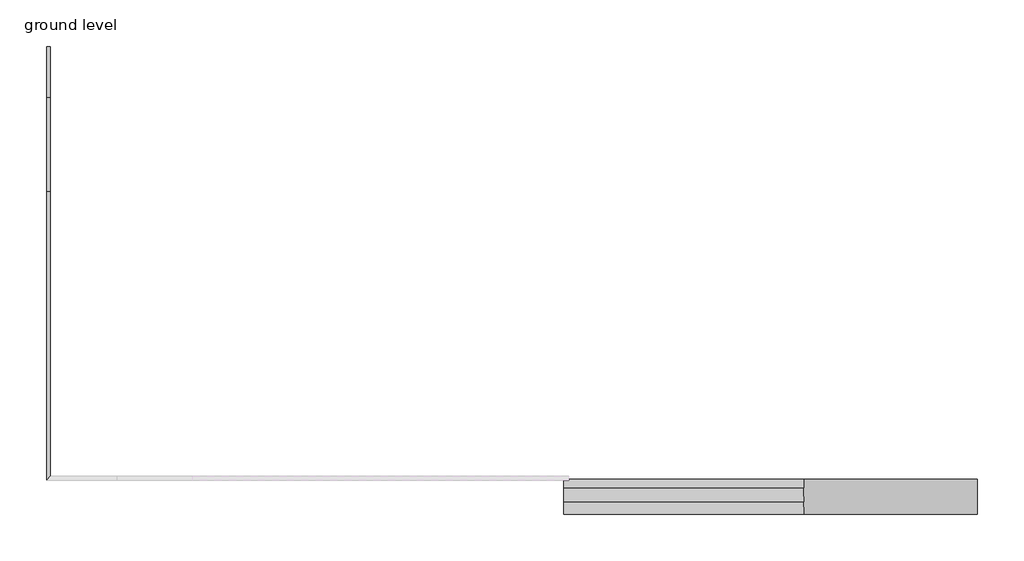
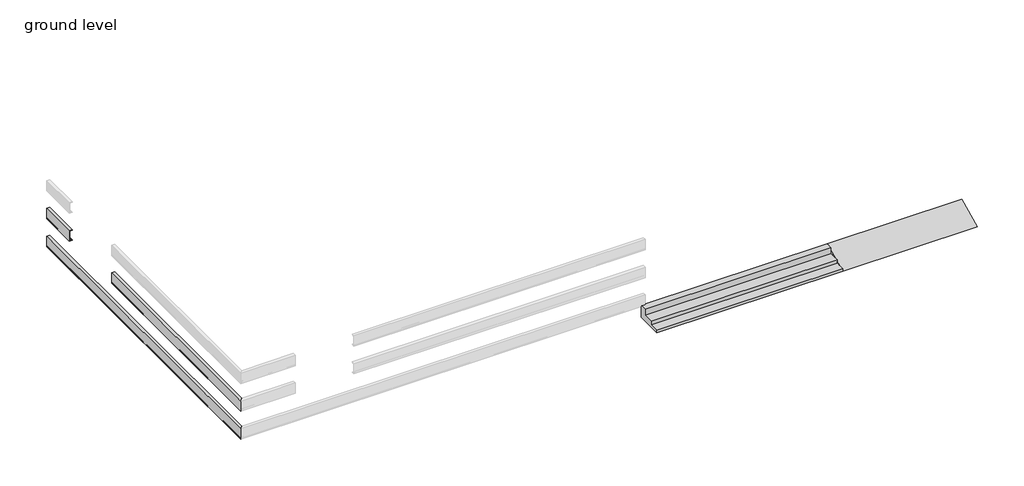
# One storey, part 3 of 3: 4 proxies.
"""IFC4 building model written with IfcOpenShell, lengths in millimetres."""

from ifc_helpers import new_model, si_unit, frame, origin, place, context, project, spatial, polyline, circle_curve, ellipse_curve, transform, mapped, element, save
from ifc_brep_helpers import plane_surface, cylinder_surface, revolved_surface, advanced_brep
from components import generic_models_3_generic_models_3_935cad4b, generic_models_4_generic_models_4_8b3ef071

model = new_model("IFC4")

# Units and contexts
model_context = context("Model", 3, world=origin())
ifc_project = project(units=[si_unit("LENGTHUNIT", "METRE", prefix="MILLI")], contexts=[model_context])

# Site, building, storey
site = spatial("IfcSite", under=ifc_project)
building = spatial("IfcBuilding", under=site)
storey = spatial("IfcBuildingStorey", under=building, Name="ground level", Elevation=0.0)

# Proxies
placement = place(None, origin())
generic_models_3_generic_models_3_shape = generic_models_3_generic_models_3_935cad4b(model_context)
element("IfcBuildingElementProxy", 1, Name="Generic Models 3 : Generic Models 3", ObjectType="Generic Models 3 : Generic Models 3", at=placement, inside=storey, context=model_context, shape_type="MappedRepresentation", body=[
    mapped(generic_models_3_generic_models_3_shape, transform((0.0, 0.0, 0.0), x_axis=(1.0, 0.0, 0.0), y_axis=(0.0, 1.0, 0.0), z_axis=(0.0, 0.0, 1.0))),
])
generic_models_4_generic_models_4_shape = generic_models_4_generic_models_4_8b3ef071(model_context)
element("IfcBuildingElementProxy", 2, Name="Generic Models 4 : Generic Models 4", ObjectType="Generic Models 4 : Generic Models 4", at=placement, inside=storey, context=model_context, shape_type="MappedRepresentation", body=[
    mapped(generic_models_4_generic_models_4_shape, transform((0.0, 0.0, 0.0), x_axis=(1.0, 0.0, 0.0), y_axis=(0.0, 1.0, 0.0), z_axis=(0.0, 0.0, 1.0))),
])
element("IfcBuildingElementProxy", 3, Name="Reveal", ObjectType="Reveal", at=placement, inside=storey, context=model_context, shape_type="AdvancedBrep", body=[
    advanced_brep(
    [(-10842.2672301, -7280.1146427, 1079.5), (-10842.2672301, -7216.8686427, 1079.5), (-10842.2672301, -7216.8686427, 1078.1203242), (-10842.2672301, -7221.2514519, 1072.9465897), (-10842.2672301, -7244.8721427, 1069.0098), (-10842.2672301, -7264.1100243, 1065.80348), (-10842.2672301, -7272.8756427, 1055.456011), (-10842.2672301, -7272.8756427, 874.943989), (-10842.2672301, -7264.1100243, 864.59652), (-10842.2672301, -7244.8721427, 861.3902), (-10842.2672301, -7221.2514519, 857.4534103), (-10842.2672301, -7216.8686427, 852.2796758), (-10842.2672301, -7216.8686427, 850.9), (-10842.2672301, -7280.1146427, 850.9), (-4797.0672301, -7280.1146427, 1079.5), (-4797.0672301, -7280.1146427, 850.9), (-4797.0672301, -7216.8686427, 850.9), (-4797.0672301, -7216.8686427, 852.2796758), (-4797.0672301, -7221.2514519, 857.4534103), (-4797.0672301, -7244.8721427, 861.3902), (-4797.0672301, -7264.1100243, 864.59652), (-4797.0672301, -7272.8756427, 874.943989), (-4797.0672301, -7272.8756427, 1055.456011), (-4797.0672301, -7264.1100243, 1065.80348), (-4797.0672301, -7244.8721427, 1069.0098), (-4797.0672301, -7221.2514519, 1072.9465897), (-4797.0672301, -7216.8686427, 1078.1203242), (-4797.0672301, -7216.8686427, 1079.5)],
    [
        (0, 1),
        (1, 2),
        (2, 3, circle_curve(frame((-10842.2672301, -7222.1137427, 1078.1203242), z_axis=(-1.0, 0.0, 0.0), x_axis=(0.0, 1.0, 0.0)), 5.2451)),
        (3, 4),
        (4, 5),
        (5, 6, circle_curve(frame((-10842.2672301, -7262.3854427, 1055.456011), z_axis=(1.0, 0.0, 0.0), x_axis=(0.0, 1.0, 0.0)), 10.4902)),
        (6, 7),
        (7, 8, circle_curve(frame((-10842.2672301, -7262.3854427, 874.943989), z_axis=(1.0, 0.0, 0.0), x_axis=(0.0, 1.0, 0.0)), 10.4902)),
        (8, 9),
        (9, 10),
        (10, 11, circle_curve(frame((-10842.2672301, -7222.1137427, 852.2796758), z_axis=(-1.0, 0.0, 0.0), x_axis=(0.0, 1.0, 0.0)), 5.2451)),
        (11, 12),
        (12, 13),
        (13, 0),
        (14, 15),
        (15, 16),
        (16, 17),
        (17, 18, circle_curve(frame((-4797.0672301, -7222.1137427, 852.2796758), z_axis=(1.0, 0.0, 0.0), x_axis=(0.0, 1.0, 0.0)), 5.2451)),
        (18, 19),
        (19, 20),
        (20, 21, circle_curve(frame((-4797.0672301, -7262.3854427, 874.943989), z_axis=(-1.0, 0.0, 0.0), x_axis=(0.0, 1.0, 0.0)), 10.4902)),
        (21, 22),
        (22, 23, circle_curve(frame((-4797.0672301, -7262.3854427, 1055.456011), z_axis=(-1.0, 0.0, 0.0), x_axis=(0.0, 1.0, 0.0)), 10.4902)),
        (23, 24),
        (24, 25),
        (25, 26, circle_curve(frame((-4797.0672301, -7222.1137427, 1078.1203242), z_axis=(1.0, 0.0, 0.0), x_axis=(0.0, 1.0, 0.0)), 5.2451)),
        (26, 27),
        (27, 14),
        (0, 14),
        (27, 1),
        (26, 2),
        (25, 3),
        (24, 4),
        (23, 5),
        (22, 6),
        (21, 7),
        (20, 8),
        (19, 9),
        (18, 10),
        (17, 11),
        (16, 12),
        (15, 13),
    ],
    [
        plane_surface(frame((-10842.2672301, -7036.6302427, 914.4), z_axis=(-1.0, 0.0, 0.0), x_axis=(0.0, -1.0, 0.0))),
        plane_surface(frame((-4797.0672301, -7265.2302427, 841.0898298), z_axis=(1.0, 0.0, 0.0), x_axis=(0.0, 1.0, 0.0))),
        plane_surface(frame((-10842.2672301, -7280.1146427, 1079.5), z_axis=(0.0, 0.0, 1.0), x_axis=(1.0, 0.0, 0.0))),
        plane_surface(frame((-10842.2672301, -7216.8686427, 1079.5), z_axis=(0.0, 1.0, 0.0), x_axis=(1.0, 0.0, 0.0))),
        cylinder_surface(frame((-10842.2672301, -7222.1137427, 1078.1203242), z_axis=(-1.0, 0.0, 0.0), x_axis=(0.0, 1.0, 0.0)), 5.2451),
        plane_surface(frame((-10842.2672301, -7221.2514519, 1072.9465897), z_axis=(0.0, 0.16439930721687082, -0.9863938705135049), x_axis=(1.0, 0.0, 0.0))),
        plane_surface(frame((-10842.2672301, -7244.8721427, 1069.0098), z_axis=(0.0, 0.16439930721687146, -0.9863938705135048), x_axis=(1.0, 0.0, 0.0))),
        revolved_surface(polyline([(-4797.0672301, -7251.8952426999995, 1055.456011), (-10842.2672301, -7251.8952426999995, 1055.456011)]), (-10842.2672301, -7262.3854427, 1055.456011), (1.0, 0.0, 0.0)),
        plane_surface(frame((-10842.2672301, -7272.8756427, 1055.456011), z_axis=(0.0, 1.0, 0.0), x_axis=(1.0, 0.0, 0.0))),
        revolved_surface(polyline([(-4797.0672301, -7251.8952426999995, 874.943989), (-10842.2672301, -7251.8952426999995, 874.943989)]), (-10842.2672301, -7262.3854427, 874.943989), (1.0, 0.0, 0.0)),
        plane_surface(frame((-10842.2672301, -7264.1100243, 864.59652), z_axis=(0.0, 0.1643993072168769, 0.9863938705135039), x_axis=(1.0, 0.0, 0.0))),
        plane_surface(frame((-10842.2672301, -7244.8721427, 861.3902), z_axis=(0.0, 0.16439930721687793, 0.9863938705135037), x_axis=(1.0, 0.0, 0.0))),
        cylinder_surface(frame((-10842.2672301, -7222.1137427, 852.2796758), z_axis=(-1.0, 0.0, 0.0), x_axis=(0.0, 1.0, 0.0)), 5.2451),
        plane_surface(frame((-10842.2672301, -7216.8686427, 852.2796758), z_axis=(0.0, 1.0, 0.0), x_axis=(1.0, 0.0, 0.0))),
        plane_surface(frame((-10842.2672301, -7216.8686427, 850.9), z_axis=(0.0, 0.0, -1.0), x_axis=(1.0, 0.0, 0.0))),
        plane_surface(frame((-10842.2672301, -7280.1146427, 850.9), z_axis=(0.0, -1.0, 0.0), x_axis=(1.0, 0.0, 0.0))),
    ],
    [
        (0, [[1, 2, 3, 4, 5, 6, 7, 8, 9, 10, 11, 12, 13, 14]]),
        (1, [[15, 16, 17, 18, 19, 20, 21, 22, 23, 24, 25, 26, 27, 28]]),
        (2, [[-1, 29, -28, 30]]),
        (3, [[-2, -30, -27, 31]]),
        (4, [[-3, -31, -26, 32]]),
        (5, [[-4, -32, -25, 33]]),
        (6, [[-5, -33, -24, 34]]),
        (7, [[-6, -34, -23, 35]]),
        (8, [[-7, -35, -22, 36]]),
        (9, [[-8, -36, -21, 37]]),
        (10, [[-9, -37, -20, 38]]),
        (11, [[-10, -38, -19, 39]]),
        (12, [[-11, -39, -18, 40]]),
        (13, [[-12, -40, -17, 41]]),
        (14, [[-13, -41, -16, 42]]),
        (15, [[-14, -42, -15, -29]]),
    ],
),
    advanced_brep(
    [(-13193.9516301, -7280.1146427, 1079.5), (-13130.7056301, -7216.8686427, 1079.5), (-13130.7056301, -7216.8686427, 1078.1203242), (-13135.0884393, -7221.2514519, 1072.9465897), (-13158.7091301, -7244.8721427, 1069.0098), (-13177.9470117, -7264.1100243, 1065.80348), (-13186.7126301, -7272.8756427, 1055.456011), (-13186.7126301, -7272.8756427, 874.943989), (-13177.9470117, -7264.1100243, 864.59652), (-13158.7091301, -7244.8721427, 861.3902), (-13135.0884393, -7221.2514519, 857.4534103), (-13130.7056301, -7216.8686427, 852.2796758), (-13130.7056301, -7216.8686427, 850.9), (-13193.9516301, -7280.1146427, 850.9), (-12061.4672301, -7280.1146427, 1079.5), (-12061.4672301, -7280.1146427, 850.9), (-12061.4672301, -7216.8686427, 850.9), (-12061.4672301, -7216.8686427, 852.2796758), (-12061.4672301, -7221.2514519, 857.4534103), (-12061.4672301, -7244.8721427, 861.3902), (-12061.4672301, -7264.1100243, 864.59652), (-12061.4672301, -7272.8756427, 874.943989), (-12061.4672301, -7272.8756427, 1055.456011), (-12061.4672301, -7264.1100243, 1065.80348), (-12061.4672301, -7244.8721427, 1069.0098), (-12061.4672301, -7221.2514519, 1072.9465897), (-12061.4672301, -7216.8686427, 1078.1203242), (-12061.4672301, -7216.8686427, 1079.5)],
    [
        (0, 1),
        (1, 2),
        (2, 3, ellipse_curve(frame((-13135.9507301, -7222.1137427, 1078.1203242), z_axis=(-0.7071067811865476, 0.7071067811865476, 0.0), x_axis=(-0.7071067811865475, -0.7071067811865476, 0.0)), 7.4176916, 5.2451)),
        (3, 4),
        (4, 5),
        (5, 6, ellipse_curve(frame((-13176.2224301, -7262.3854427, 1055.456011), z_axis=(0.7071067811865476, -0.7071067811865476, 0.0), x_axis=(0.7071067811865475, 0.7071067811865476, 0.0)), 14.8353831, 10.4902)),
        (6, 7),
        (7, 8, ellipse_curve(frame((-13176.2224301, -7262.3854427, 874.943989), z_axis=(0.7071067811865476, -0.7071067811865476, 0.0), x_axis=(0.7071067811865475, 0.7071067811865476, 0.0)), 14.8353831, 10.4902)),
        (8, 9),
        (9, 10),
        (10, 11, ellipse_curve(frame((-13135.9507301, -7222.1137427, 852.2796758), z_axis=(-0.7071067811865476, 0.7071067811865476, 0.0), x_axis=(-0.7071067811865475, -0.7071067811865476, 0.0)), 7.4176916, 5.2451)),
        (11, 12),
        (12, 13),
        (13, 0),
        (14, 15),
        (15, 16),
        (16, 17),
        (17, 18, circle_curve(frame((-12061.4672301, -7222.1137427, 852.2796758), z_axis=(1.0, 0.0, 0.0), x_axis=(0.0, 1.0, 0.0)), 5.2451)),
        (18, 19),
        (19, 20),
        (20, 21, circle_curve(frame((-12061.4672301, -7262.3854427, 874.943989), z_axis=(-1.0, 0.0, 0.0), x_axis=(0.0, 1.0, 0.0)), 10.4902)),
        (21, 22),
        (22, 23, circle_curve(frame((-12061.4672301, -7262.3854427, 1055.456011), z_axis=(-1.0, 0.0, 0.0), x_axis=(0.0, 1.0, 0.0)), 10.4902)),
        (23, 24),
        (24, 25),
        (25, 26, circle_curve(frame((-12061.4672301, -7222.1137427, 1078.1203242), z_axis=(1.0, 0.0, 0.0), x_axis=(0.0, 1.0, 0.0)), 5.2451)),
        (26, 27),
        (27, 14),
        (0, 14),
        (27, 1),
        (26, 2),
        (25, 3),
        (24, 4),
        (23, 5),
        (22, 6),
        (21, 7),
        (20, 8),
        (19, 9),
        (18, 10),
        (17, 11),
        (16, 12),
        (15, 13),
    ],
    [
        plane_surface(frame((-13179.0672301, -7265.2302427, 660.4), z_axis=(-0.7071067811865476, 0.7071067811865476, 0.0), x_axis=(0.7071067811865476, 0.7071067811865476, 0.0))),
        plane_surface(frame((-12061.4672301, -7036.6302427, 2184.4), z_axis=(1.0, 0.0, 0.0), x_axis=(0.0, -1.0, 0.0))),
        plane_surface(frame((-13193.9516301, -7280.1146427, 1079.5), z_axis=(0.0, 0.0, 1.0), x_axis=(1.0, 0.0, 0.0))),
        plane_surface(frame((-13130.7056301, -7216.8686427, 1079.5), z_axis=(0.0, 1.0, 0.0), x_axis=(1.0, 0.0, 0.0))),
        cylinder_surface(frame((-13179.0672301, -7222.1137427, 1078.1203242), z_axis=(-1.0, 0.0, 0.0), x_axis=(0.0, 1.0, 0.0)), 5.2451),
        plane_surface(frame((-13135.0884393, -7221.2514519, 1072.9465897), z_axis=(0.0, 0.16439930721687082, -0.9863938705135049), x_axis=(1.0, 0.0, 0.0))),
        plane_surface(frame((-13158.7091301, -7244.8721427, 1069.0098), z_axis=(0.0, 0.16439930721687146, -0.9863938705135048), x_axis=(1.0, 0.0, 0.0))),
        revolved_surface(polyline([(-12061.4672301, -7251.8952426999995, 1055.456011), (-13186.7126301, -7251.8952426999995, 1055.456011)]), (-13179.0672301, -7262.3854427, 1055.456011), (1.0, 0.0, 0.0)),
        plane_surface(frame((-13186.7126301, -7272.8756427, 1055.456011), z_axis=(0.0, 1.0, 0.0), x_axis=(1.0, 0.0, 0.0))),
        revolved_surface(polyline([(-12061.4672301, -7251.8952426999995, 874.943989), (-13186.7126301, -7251.8952426999995, 874.943989)]), (-13179.0672301, -7262.3854427, 874.943989), (1.0, 0.0, 0.0)),
        plane_surface(frame((-13177.9470117, -7264.1100243, 864.59652), z_axis=(0.0, 0.1643993072168769, 0.9863938705135039), x_axis=(1.0, 0.0, 0.0))),
        plane_surface(frame((-13158.7091301, -7244.8721427, 861.3902), z_axis=(0.0, 0.16439930721687793, 0.9863938705135037), x_axis=(1.0, 0.0, 0.0))),
        cylinder_surface(frame((-13179.0672301, -7222.1137427, 852.2796758), z_axis=(-1.0, 0.0, 0.0), x_axis=(0.0, 1.0, 0.0)), 5.2451),
        plane_surface(frame((-13130.7056301, -7216.8686427, 852.2796758), z_axis=(0.0, 1.0, 0.0), x_axis=(1.0, 0.0, 0.0))),
        plane_surface(frame((-13130.7056301, -7216.8686427, 850.9), z_axis=(0.0, 0.0, -1.0), x_axis=(1.0, 0.0, 0.0))),
        plane_surface(frame((-13193.9516301, -7280.1146427, 850.9), z_axis=(0.0, -1.0, 0.0), x_axis=(1.0, 0.0, 0.0))),
    ],
    [
        (0, [[1, 2, 3, 4, 5, 6, 7, 8, 9, 10, 11, 12, 13, 14]]),
        (1, [[15, 16, 17, 18, 19, 20, 21, 22, 23, 24, 25, 26, 27, 28]]),
        (2, [[-1, 29, -28, 30]]),
        (3, [[-2, -30, -27, 31]]),
        (4, [[-3, -31, -26, 32]]),
        (5, [[-4, -32, -25, 33]]),
        (6, [[-5, -33, -24, 34]]),
        (7, [[-6, -34, -23, 35]]),
        (8, [[-7, -35, -22, 36]]),
        (9, [[-8, -36, -21, 37]]),
        (10, [[-9, -37, -20, 38]]),
        (11, [[-10, -38, -19, 39]]),
        (12, [[-11, -39, -18, 40]]),
        (13, [[-12, -40, -17, 41]]),
        (14, [[-13, -41, -16, 42]]),
        (15, [[-14, -42, -15, -29]]),
    ],
),
    advanced_brep(
    [(-13193.9516301, -2642.4302427, 1079.5), (-13130.7056301, -2642.4302427, 1079.5), (-13130.7056301, -2642.4302427, 1078.1203242), (-13135.0884393, -2642.4302427, 1072.9465897), (-13158.7091301, -2642.4302427, 1069.0098), (-13177.9470117, -2642.4302427, 1065.80348), (-13186.7126301, -2642.4302427, 1055.456011), (-13186.7126301, -2642.4302427, 874.943989), (-13177.9470117, -2642.4302427, 864.59652), (-13158.7091301, -2642.4302427, 861.3902), (-13135.0884393, -2642.4302427, 857.4534103), (-13130.7056301, -2642.4302427, 852.2796758), (-13130.7056301, -2642.4302427, 850.9), (-13193.9516301, -2642.4302427, 850.9), (-13193.9516301, -7280.1146427, 1079.5), (-13193.9516301, -7280.1146427, 850.9), (-13130.7056301, -7216.8686427, 850.9), (-13130.7056301, -7216.8686427, 852.2796758), (-13135.0884393, -7221.2514519, 857.4534103), (-13158.7091301, -7244.8721427, 861.3902), (-13177.9470117, -7264.1100243, 864.59652), (-13186.7126301, -7272.8756427, 874.943989), (-13186.7126301, -7272.8756427, 1055.456011), (-13177.9470117, -7264.1100243, 1065.80348), (-13158.7091301, -7244.8721427, 1069.0098), (-13135.0884393, -7221.2514519, 1072.9465897), (-13130.7056301, -7216.8686427, 1078.1203242), (-13130.7056301, -7216.8686427, 1079.5)],
    [
        (0, 1),
        (1, 2),
        (2, 3, circle_curve(frame((-13135.9507301, -2642.4302427, 1078.1203242), z_axis=(0.0, 1.0, 0.0), x_axis=(1.0, 0.0, 0.0)), 5.2451)),
        (3, 4),
        (4, 5),
        (5, 6, circle_curve(frame((-13176.2224301, -2642.4302427, 1055.456011), z_axis=(0.0, -1.0, 0.0), x_axis=(1.0, 0.0, 0.0)), 10.4902)),
        (6, 7),
        (7, 8, circle_curve(frame((-13176.2224301, -2642.4302427, 874.943989), z_axis=(0.0, -1.0, 0.0), x_axis=(1.0, 0.0, 0.0)), 10.4902)),
        (8, 9),
        (9, 10),
        (10, 11, circle_curve(frame((-13135.9507301, -2642.4302427, 852.2796758), z_axis=(0.0, 1.0, 0.0), x_axis=(1.0, 0.0, 0.0)), 5.2451)),
        (11, 12),
        (12, 13),
        (13, 0),
        (14, 15),
        (15, 16),
        (16, 17),
        (17, 18, ellipse_curve(frame((-13135.9507301, -7222.1137427, 852.2796758), z_axis=(0.7071067811865476, -0.7071067811865476, 0.0), x_axis=(0.7071067811865477, 0.7071067811865474, 0.0)), 7.4176916, 5.2451)),
        (18, 19),
        (19, 20),
        (20, 21, ellipse_curve(frame((-13176.2224301, -7262.3854427, 874.943989), z_axis=(-0.7071067811865476, 0.7071067811865476, 0.0), x_axis=(-0.7071067811865477, -0.7071067811865474, 0.0)), 14.8353831, 10.4902)),
        (21, 22),
        (22, 23, ellipse_curve(frame((-13176.2224301, -7262.3854427, 1055.456011), z_axis=(-0.7071067811865476, 0.7071067811865476, 0.0), x_axis=(-0.7071067811865477, -0.7071067811865474, 0.0)), 14.8353831, 10.4902)),
        (23, 24),
        (24, 25),
        (25, 26, ellipse_curve(frame((-13135.9507301, -7222.1137427, 1078.1203242), z_axis=(0.7071067811865476, -0.7071067811865476, 0.0), x_axis=(0.7071067811865477, 0.7071067811865474, 0.0)), 7.4176916, 5.2451)),
        (26, 27),
        (27, 14),
        (0, 14),
        (27, 1),
        (26, 2),
        (25, 3),
        (24, 4),
        (23, 5),
        (22, 6),
        (21, 7),
        (20, 8),
        (19, 9),
        (18, 10),
        (17, 11),
        (16, 12),
        (15, 13),
    ],
    [
        plane_surface(frame((-12950.4672301, -2642.4302427, 914.4), z_axis=(0.0, 1.0, 0.0), x_axis=(-1.0, 0.0, 0.0))),
        plane_surface(frame((-13179.0672301, -7265.2302427, 660.4), z_axis=(0.7071067811865476, -0.7071067811865476, 0.0), x_axis=(0.7071067811865476, 0.7071067811865476, 0.0))),
        plane_surface(frame((-13193.9516301, -2642.4302427, 1079.5), z_axis=(0.0, 0.0, 1.0), x_axis=(0.0, -1.0, 0.0))),
        plane_surface(frame((-13130.7056301, -2642.4302427, 1079.5), z_axis=(1.0, 0.0, 0.0), x_axis=(0.0, -1.0, 0.0))),
        cylinder_surface(frame((-13135.9507301, -2642.4302427, 1078.1203242), z_axis=(0.0, 1.0, 0.0), x_axis=(1.0, 0.0, 0.0)), 5.2451),
        plane_surface(frame((-13135.0884393, -2642.4302427, 1072.9465897), z_axis=(0.16439930721687082, 0.0, -0.9863938705135049), x_axis=(0.0, -1.0, 0.0))),
        plane_surface(frame((-13158.7091301, -2642.4302427, 1069.0098), z_axis=(0.16439930721687146, 0.0, -0.9863938705135048), x_axis=(0.0, -1.0, 0.0))),
        revolved_surface(polyline([(-13165.7322301, -7272.875642700001, 1055.456011), (-13165.7322301, -2642.4302427, 1055.456011)]), (-13176.2224301, -2642.4302427, 1055.456011), (0.0, -1.0, 0.0)),
        plane_surface(frame((-13186.7126301, -2642.4302427, 1055.456011), z_axis=(1.0, 0.0, 0.0), x_axis=(0.0, -1.0, 0.0))),
        revolved_surface(polyline([(-13165.7322301, -7272.875642700001, 874.943989), (-13165.7322301, -2642.4302427, 874.943989)]), (-13176.2224301, -2642.4302427, 874.943989), (0.0, -1.0, 0.0)),
        plane_surface(frame((-13177.9470117, -2642.4302427, 864.59652), z_axis=(0.1643993072168769, 0.0, 0.9863938705135039), x_axis=(0.0, -1.0, 0.0))),
        plane_surface(frame((-13158.7091301, -2642.4302427, 861.3902), z_axis=(0.16439930721687793, 0.0, 0.9863938705135037), x_axis=(0.0, -1.0, 0.0))),
        cylinder_surface(frame((-13135.9507301, -2642.4302427, 852.2796758), z_axis=(0.0, 1.0, 0.0), x_axis=(1.0, 0.0, 0.0)), 5.2451),
        plane_surface(frame((-13130.7056301, -2642.4302427, 852.2796758), z_axis=(1.0, 0.0, 0.0), x_axis=(0.0, -1.0, 0.0))),
        plane_surface(frame((-13130.7056301, -2642.4302427, 850.9), z_axis=(0.0, 0.0, -1.0), x_axis=(0.0, -1.0, 0.0))),
        plane_surface(frame((-13193.9516301, -2642.4302427, 850.9), z_axis=(-1.0, 0.0, 0.0), x_axis=(0.0, -1.0, 0.0))),
    ],
    [
        (0, [[1, 2, 3, 4, 5, 6, 7, 8, 9, 10, 11, 12, 13, 14]]),
        (1, [[15, 16, 17, 18, 19, 20, 21, 22, 23, 24, 25, 26, 27, 28]]),
        (2, [[-1, 29, -28, 30]]),
        (3, [[-2, -30, -27, 31]]),
        (4, [[-3, -31, -26, 32]]),
        (5, [[-4, -32, -25, 33]]),
        (6, [[-5, -33, -24, 34]]),
        (7, [[-6, -34, -23, 35]]),
        (8, [[-7, -35, -22, 36]]),
        (9, [[-8, -36, -21, 37]]),
        (10, [[-9, -37, -20, 38]]),
        (11, [[-10, -38, -19, 39]]),
        (12, [[-11, -39, -18, 40]]),
        (13, [[-12, -40, -17, 41]]),
        (14, [[-13, -41, -16, 42]]),
        (15, [[-14, -42, -15, -29]]),
    ],
),
    advanced_brep(
    [(-13193.9516301, -305.6302427, 1079.5), (-13130.7056301, -305.6302427, 1079.5), (-13130.7056301, -305.6302427, 1078.1203242), (-13135.0884393, -305.6302427, 1072.9465897), (-13158.7091301, -305.6302427, 1069.0098), (-13177.9470117, -305.6302427, 1065.80348), (-13186.7126301, -305.6302427, 1055.456011), (-13186.7126301, -305.6302427, 874.943989), (-13177.9470117, -305.6302427, 864.59652), (-13158.7091301, -305.6302427, 861.3902), (-13135.0884393, -305.6302427, 857.4534103), (-13130.7056301, -305.6302427, 852.2796758), (-13130.7056301, -305.6302427, 850.9), (-13193.9516301, -305.6302427, 850.9), (-13193.9516301, -1118.4302427, 1079.5), (-13193.9516301, -1118.4302427, 850.9), (-13130.7056301, -1118.4302427, 850.9), (-13130.7056301, -1118.4302427, 852.2796758), (-13135.0884393, -1118.4302427, 857.4534103), (-13158.7091301, -1118.4302427, 861.3902), (-13177.9470117, -1118.4302427, 864.59652), (-13186.7126301, -1118.4302427, 874.943989), (-13186.7126301, -1118.4302427, 1055.456011), (-13177.9470117, -1118.4302427, 1065.80348), (-13158.7091301, -1118.4302427, 1069.0098), (-13135.0884393, -1118.4302427, 1072.9465897), (-13130.7056301, -1118.4302427, 1078.1203242), (-13130.7056301, -1118.4302427, 1079.5)],
    [
        (0, 1),
        (1, 2),
        (2, 3, circle_curve(frame((-13135.9507301, -305.6302427, 1078.1203242), z_axis=(0.0, 1.0, 0.0), x_axis=(1.0, 0.0, 0.0)), 5.2451)),
        (3, 4),
        (4, 5),
        (5, 6, circle_curve(frame((-13176.2224301, -305.6302427, 1055.456011), z_axis=(0.0, -1.0, 0.0), x_axis=(1.0, 0.0, 0.0)), 10.4902)),
        (6, 7),
        (7, 8, circle_curve(frame((-13176.2224301, -305.6302427, 874.943989), z_axis=(0.0, -1.0, 0.0), x_axis=(1.0, 0.0, 0.0)), 10.4902)),
        (8, 9),
        (9, 10),
        (10, 11, circle_curve(frame((-13135.9507301, -305.6302427, 852.2796758), z_axis=(0.0, 1.0, 0.0), x_axis=(1.0, 0.0, 0.0)), 5.2451)),
        (11, 12),
        (12, 13),
        (13, 0),
        (14, 15),
        (15, 16),
        (16, 17),
        (17, 18, circle_curve(frame((-13135.9507301, -1118.4302427, 852.2796758), z_axis=(0.0, -1.0, 0.0), x_axis=(1.0, 0.0, 0.0)), 5.2451)),
        (18, 19),
        (19, 20),
        (20, 21, circle_curve(frame((-13176.2224301, -1118.4302427, 874.943989), z_axis=(0.0, 1.0, 0.0), x_axis=(1.0, 0.0, 0.0)), 10.4902)),
        (21, 22),
        (22, 23, circle_curve(frame((-13176.2224301, -1118.4302427, 1055.456011), z_axis=(0.0, 1.0, 0.0), x_axis=(1.0, 0.0, 0.0)), 10.4902)),
        (23, 24),
        (24, 25),
        (25, 26, circle_curve(frame((-13135.9507301, -1118.4302427, 1078.1203242), z_axis=(0.0, -1.0, 0.0), x_axis=(1.0, 0.0, 0.0)), 5.2451)),
        (26, 27),
        (27, 14),
        (0, 14),
        (27, 1),
        (26, 2),
        (25, 3),
        (24, 4),
        (23, 5),
        (22, 6),
        (21, 7),
        (20, 8),
        (19, 9),
        (18, 10),
        (17, 11),
        (16, 12),
        (15, 13),
    ],
    [
        plane_surface(frame((-12942.6830845, -305.6302427, 304.8), z_axis=(0.0, 1.0, 0.0), x_axis=(-1.0, 0.0, 0.0))),
        plane_surface(frame((-12950.4672301, -1118.4302427, 2489.2), z_axis=(0.0, -1.0, 0.0), x_axis=(-1.0, 0.0, 0.0))),
        plane_surface(frame((-13193.9516301, -305.6302427, 1079.5), z_axis=(0.0, 0.0, 1.0), x_axis=(0.0, -1.0, 0.0))),
        plane_surface(frame((-13130.7056301, -305.6302427, 1079.5), z_axis=(1.0, 0.0, 0.0), x_axis=(0.0, -1.0, 0.0))),
        cylinder_surface(frame((-13135.9507301, -305.6302427, 1078.1203242), z_axis=(0.0, 1.0, 0.0), x_axis=(1.0, 0.0, 0.0)), 5.2451),
        plane_surface(frame((-13135.0884393, -305.6302427, 1072.9465897), z_axis=(0.16439930721687082, 0.0, -0.9863938705135049), x_axis=(0.0, -1.0, 0.0))),
        plane_surface(frame((-13158.7091301, -305.6302427, 1069.0098), z_axis=(0.16439930721687146, 0.0, -0.9863938705135048), x_axis=(0.0, -1.0, 0.0))),
        revolved_surface(polyline([(-13165.7322301, -1118.4302427, 1055.456011), (-13165.7322301, -305.6302427, 1055.456011)]), (-13176.2224301, -305.6302427, 1055.456011), (0.0, -1.0, 0.0)),
        plane_surface(frame((-13186.7126301, -305.6302427, 1055.456011), z_axis=(1.0, 0.0, 0.0), x_axis=(0.0, -1.0, 0.0))),
        revolved_surface(polyline([(-13165.7322301, -1118.4302427, 874.943989), (-13165.7322301, -305.6302427, 874.943989)]), (-13176.2224301, -305.6302427, 874.943989), (0.0, -1.0, 0.0)),
        plane_surface(frame((-13177.9470117, -305.6302427, 864.59652), z_axis=(0.1643993072168769, 0.0, 0.9863938705135039), x_axis=(0.0, -1.0, 0.0))),
        plane_surface(frame((-13158.7091301, -305.6302427, 861.3902), z_axis=(0.16439930721687793, 0.0, 0.9863938705135037), x_axis=(0.0, -1.0, 0.0))),
        cylinder_surface(frame((-13135.9507301, -305.6302427, 852.2796758), z_axis=(0.0, 1.0, 0.0), x_axis=(1.0, 0.0, 0.0)), 5.2451),
        plane_surface(frame((-13130.7056301, -305.6302427, 852.2796758), z_axis=(1.0, 0.0, 0.0), x_axis=(0.0, -1.0, 0.0))),
        plane_surface(frame((-13130.7056301, -305.6302427, 850.9), z_axis=(0.0, 0.0, -1.0), x_axis=(0.0, -1.0, 0.0))),
        plane_surface(frame((-13193.9516301, -305.6302427, 850.9), z_axis=(-1.0, 0.0, 0.0), x_axis=(0.0, -1.0, 0.0))),
    ],
    [
        (0, [[1, 2, 3, 4, 5, 6, 7, 8, 9, 10, 11, 12, 13, 14]]),
        (1, [[15, 16, 17, 18, 19, 20, 21, 22, 23, 24, 25, 26, 27, 28]]),
        (2, [[-1, 29, -28, 30]]),
        (3, [[-2, -30, -27, 31]]),
        (4, [[-3, -31, -26, 32]]),
        (5, [[-4, -32, -25, 33]]),
        (6, [[-5, -33, -24, 34]]),
        (7, [[-6, -34, -23, 35]]),
        (8, [[-7, -35, -22, 36]]),
        (9, [[-8, -36, -21, 37]]),
        (10, [[-9, -37, -20, 38]]),
        (11, [[-10, -38, -19, 39]]),
        (12, [[-11, -39, -18, 40]]),
        (13, [[-12, -40, -17, 41]]),
        (14, [[-13, -41, -16, 42]]),
        (15, [[-14, -42, -15, -29]]),
    ],
),
])
element("IfcBuildingElementProxy", 4, Name="Reveal", ObjectType="Reveal", at=placement, inside=storey, context=model_context, shape_type="AdvancedBrep", body=[
    advanced_brep(
    [(-13193.9516301, -7280.1146427, 469.9), (-13130.7056301, -7216.8686427, 469.9), (-13130.7056301, -7216.8686427, 468.5203242), (-13135.0884393, -7221.2514519, 463.3465897), (-13158.7091301, -7244.8721427, 459.4098), (-13177.9470117, -7264.1100243, 456.20348), (-13186.7126301, -7272.8756427, 445.856011), (-13186.7126301, -7272.8756427, 265.343989), (-13177.9470117, -7264.1100243, 254.99652), (-13158.7091301, -7244.8721427, 251.7902), (-13135.0884393, -7221.2514519, 247.8534103), (-13130.7056301, -7216.8686427, 242.6796758), (-13130.7056301, -7216.8686427, 241.3), (-13193.9516301, -7280.1146427, 241.3), (-4797.0672301, -7280.1146427, 469.9), (-4797.0672301, -7280.1146427, 241.3), (-4797.0672301, -7216.8686427, 241.3), (-4797.0672301, -7216.8686427, 242.6796758), (-4797.0672301, -7221.2514519, 247.8534103), (-4797.0672301, -7244.8721427, 251.7902), (-4797.0672301, -7264.1100243, 254.99652), (-4797.0672301, -7272.8756427, 265.343989), (-4797.0672301, -7272.8756427, 445.856011), (-4797.0672301, -7264.1100243, 456.20348), (-4797.0672301, -7244.8721427, 459.4098), (-4797.0672301, -7221.2514519, 463.3465897), (-4797.0672301, -7216.8686427, 468.5203242), (-4797.0672301, -7216.8686427, 469.9)],
    [
        (0, 1),
        (1, 2),
        (2, 3, ellipse_curve(frame((-13135.9507301, -7222.1137427, 468.5203242), z_axis=(-0.7071067811865476, 0.7071067811865476, 0.0), x_axis=(-0.7071067811865475, -0.7071067811865476, 0.0)), 7.4176916, 5.2451)),
        (3, 4),
        (4, 5),
        (5, 6, ellipse_curve(frame((-13176.2224301, -7262.3854427, 445.856011), z_axis=(0.7071067811865476, -0.7071067811865476, 0.0), x_axis=(0.7071067811865475, 0.7071067811865476, 0.0)), 14.8353831, 10.4902)),
        (6, 7),
        (7, 8, ellipse_curve(frame((-13176.2224301, -7262.3854427, 265.343989), z_axis=(0.7071067811865476, -0.7071067811865476, 0.0), x_axis=(0.7071067811865475, 0.7071067811865476, 0.0)), 14.8353831, 10.4902)),
        (8, 9),
        (9, 10),
        (10, 11, ellipse_curve(frame((-13135.9507301, -7222.1137427, 242.6796758), z_axis=(-0.7071067811865476, 0.7071067811865476, 0.0), x_axis=(-0.7071067811865475, -0.7071067811865476, 0.0)), 7.4176916, 5.2451)),
        (11, 12),
        (12, 13),
        (13, 0),
        (14, 15),
        (15, 16),
        (16, 17),
        (17, 18, circle_curve(frame((-4797.0672301, -7222.1137427, 242.6796758), z_axis=(1.0, 0.0, 0.0), x_axis=(0.0, 1.0, 0.0)), 5.2451)),
        (18, 19),
        (19, 20),
        (20, 21, circle_curve(frame((-4797.0672301, -7262.3854427, 265.343989), z_axis=(-1.0, 0.0, 0.0), x_axis=(0.0, 1.0, 0.0)), 10.4902)),
        (21, 22),
        (22, 23, circle_curve(frame((-4797.0672301, -7262.3854427, 445.856011), z_axis=(-1.0, 0.0, 0.0), x_axis=(0.0, 1.0, 0.0)), 10.4902)),
        (23, 24),
        (24, 25),
        (25, 26, circle_curve(frame((-4797.0672301, -7222.1137427, 468.5203242), z_axis=(1.0, 0.0, 0.0), x_axis=(0.0, 1.0, 0.0)), 5.2451)),
        (26, 27),
        (27, 14),
        (0, 14),
        (27, 1),
        (26, 2),
        (25, 3),
        (24, 4),
        (23, 5),
        (22, 6),
        (21, 7),
        (20, 8),
        (19, 9),
        (18, 10),
        (17, 11),
        (16, 12),
        (15, 13),
    ],
    [
        plane_surface(frame((-13179.0672301, -7265.2302427, 50.8), z_axis=(-0.7071067811865476, 0.7071067811865476, 0.0), x_axis=(0.7071067811865476, 0.7071067811865476, 0.0))),
        plane_surface(frame((-4797.0672301, -7265.2302427, 231.4898298), z_axis=(1.0, 0.0, 0.0), x_axis=(0.0, 1.0, 0.0))),
        plane_surface(frame((-13193.9516301, -7280.1146427, 469.9), z_axis=(0.0, 0.0, 1.0), x_axis=(1.0, 0.0, 0.0))),
        plane_surface(frame((-13130.7056301, -7216.8686427, 469.9), z_axis=(0.0, 1.0, 0.0), x_axis=(1.0, 0.0, 0.0))),
        cylinder_surface(frame((-13179.0672301, -7222.1137427, 468.5203242), z_axis=(-1.0, 0.0, 0.0), x_axis=(0.0, 1.0, 0.0)), 5.2451),
        plane_surface(frame((-13135.0884393, -7221.2514519, 463.3465897), z_axis=(0.0, 0.16439930721687082, -0.9863938705135049), x_axis=(1.0, 0.0, 0.0))),
        plane_surface(frame((-13158.7091301, -7244.8721427, 459.4098), z_axis=(0.0, 0.16439930721687146, -0.9863938705135048), x_axis=(1.0, 0.0, 0.0))),
        revolved_surface(polyline([(-4797.0672300999995, -7251.8952426999995, 445.856011), (-13186.7126301, -7251.8952426999995, 445.856011)]), (-13179.0672301, -7262.3854427, 445.856011), (1.0, 0.0, 0.0)),
        plane_surface(frame((-13186.7126301, -7272.8756427, 445.856011), z_axis=(0.0, 1.0, 0.0), x_axis=(1.0, 0.0, 0.0))),
        revolved_surface(polyline([(-4797.0672300999995, -7251.8952426999995, 265.343989), (-13186.7126301, -7251.8952426999995, 265.343989)]), (-13179.0672301, -7262.3854427, 265.343989), (1.0, 0.0, 0.0)),
        plane_surface(frame((-13177.9470117, -7264.1100243, 254.99652), z_axis=(0.0, 0.1643993072168769, 0.9863938705135039), x_axis=(1.0, 0.0, 0.0))),
        plane_surface(frame((-13158.7091301, -7244.8721427, 251.7902), z_axis=(0.0, 0.16439930721687793, 0.9863938705135037), x_axis=(1.0, 0.0, 0.0))),
        cylinder_surface(frame((-13179.0672301, -7222.1137427, 242.6796758), z_axis=(-1.0, 0.0, 0.0), x_axis=(0.0, 1.0, 0.0)), 5.2451),
        plane_surface(frame((-13130.7056301, -7216.8686427, 242.6796758), z_axis=(0.0, 1.0, 0.0), x_axis=(1.0, 0.0, 0.0))),
        plane_surface(frame((-13130.7056301, -7216.8686427, 241.3), z_axis=(0.0, 0.0, -1.0), x_axis=(1.0, 0.0, 0.0))),
        plane_surface(frame((-13193.9516301, -7280.1146427, 241.3), z_axis=(0.0, -1.0, 0.0), x_axis=(1.0, 0.0, 0.0))),
    ],
    [
        (0, [[1, 2, 3, 4, 5, 6, 7, 8, 9, 10, 11, 12, 13, 14]]),
        (1, [[15, 16, 17, 18, 19, 20, 21, 22, 23, 24, 25, 26, 27, 28]]),
        (2, [[-1, 29, -28, 30]]),
        (3, [[-2, -30, -27, 31]]),
        (4, [[-3, -31, -26, 32]]),
        (5, [[-4, -32, -25, 33]]),
        (6, [[-5, -33, -24, 34]]),
        (7, [[-6, -34, -23, 35]]),
        (8, [[-7, -35, -22, 36]]),
        (9, [[-8, -36, -21, 37]]),
        (10, [[-9, -37, -20, 38]]),
        (11, [[-10, -38, -19, 39]]),
        (12, [[-11, -39, -18, 40]]),
        (13, [[-12, -40, -17, 41]]),
        (14, [[-13, -41, -16, 42]]),
        (15, [[-14, -42, -15, -29]]),
    ],
),
    advanced_brep(
    [(-13193.9516301, -305.6302427, 469.9), (-13130.7056301, -305.6302427, 469.9), (-13130.7056301, -305.6302427, 468.5203242), (-13135.0884393, -305.6302427, 463.3465897), (-13158.7091301, -305.6302427, 459.4098), (-13177.9470117, -305.6302427, 456.20348), (-13186.7126301, -305.6302427, 445.856011), (-13186.7126301, -305.6302427, 265.343989), (-13177.9470117, -305.6302427, 254.99652), (-13158.7091301, -305.6302427, 251.7902), (-13135.0884393, -305.6302427, 247.8534103), (-13130.7056301, -305.6302427, 242.6796758), (-13130.7056301, -305.6302427, 241.3), (-13193.9516301, -305.6302427, 241.3), (-13193.9516301, -7280.1146427, 469.9), (-13193.9516301, -7280.1146427, 241.3), (-13130.7056301, -7216.8686427, 241.3), (-13130.7056301, -7216.8686427, 242.6796758), (-13135.0884393, -7221.2514519, 247.8534103), (-13158.7091301, -7244.8721427, 251.7902), (-13177.9470117, -7264.1100243, 254.99652), (-13186.7126301, -7272.8756427, 265.343989), (-13186.7126301, -7272.8756427, 445.856011), (-13177.9470117, -7264.1100243, 456.20348), (-13158.7091301, -7244.8721427, 459.4098), (-13135.0884393, -7221.2514519, 463.3465897), (-13130.7056301, -7216.8686427, 468.5203242), (-13130.7056301, -7216.8686427, 469.9)],
    [
        (0, 1),
        (1, 2),
        (2, 3, circle_curve(frame((-13135.9507301, -305.6302427, 468.5203242), z_axis=(0.0, 1.0, 0.0), x_axis=(1.0, 0.0, 0.0)), 5.2451)),
        (3, 4),
        (4, 5),
        (5, 6, circle_curve(frame((-13176.2224301, -305.6302427, 445.856011), z_axis=(0.0, -1.0, 0.0), x_axis=(1.0, 0.0, 0.0)), 10.4902)),
        (6, 7),
        (7, 8, circle_curve(frame((-13176.2224301, -305.6302427, 265.343989), z_axis=(0.0, -1.0, 0.0), x_axis=(1.0, 0.0, 0.0)), 10.4902)),
        (8, 9),
        (9, 10),
        (10, 11, circle_curve(frame((-13135.9507301, -305.6302427, 242.6796758), z_axis=(0.0, 1.0, 0.0), x_axis=(1.0, 0.0, 0.0)), 5.2451)),
        (11, 12),
        (12, 13),
        (13, 0),
        (14, 15),
        (15, 16),
        (16, 17),
        (17, 18, ellipse_curve(frame((-13135.9507301, -7222.1137427, 242.6796758), z_axis=(0.7071067811865476, -0.7071067811865476, 0.0), x_axis=(0.7071067811865477, 0.7071067811865474, 0.0)), 7.4176916, 5.2451)),
        (18, 19),
        (19, 20),
        (20, 21, ellipse_curve(frame((-13176.2224301, -7262.3854427, 265.343989), z_axis=(-0.7071067811865476, 0.7071067811865476, 0.0), x_axis=(-0.7071067811865477, -0.7071067811865474, 0.0)), 14.8353831, 10.4902)),
        (21, 22),
        (22, 23, ellipse_curve(frame((-13176.2224301, -7262.3854427, 445.856011), z_axis=(-0.7071067811865476, 0.7071067811865476, 0.0), x_axis=(-0.7071067811865477, -0.7071067811865474, 0.0)), 14.8353831, 10.4902)),
        (23, 24),
        (24, 25),
        (25, 26, ellipse_curve(frame((-13135.9507301, -7222.1137427, 468.5203242), z_axis=(0.7071067811865476, -0.7071067811865476, 0.0), x_axis=(0.7071067811865477, 0.7071067811865474, 0.0)), 7.4176916, 5.2451)),
        (26, 27),
        (27, 14),
        (0, 14),
        (27, 1),
        (26, 2),
        (25, 3),
        (24, 4),
        (23, 5),
        (22, 6),
        (21, 7),
        (20, 8),
        (19, 9),
        (18, 10),
        (17, 11),
        (16, 12),
        (15, 13),
    ],
    [
        plane_surface(frame((-12942.6830845, -305.6302427, 304.8), z_axis=(0.0, 1.0, 0.0), x_axis=(-1.0, 0.0, 0.0))),
        plane_surface(frame((-13179.0672301, -7265.2302427, 50.8), z_axis=(0.7071067811865476, -0.7071067811865476, 0.0), x_axis=(0.7071067811865476, 0.7071067811865476, 0.0))),
        plane_surface(frame((-13193.9516301, -305.6302427, 469.9), z_axis=(0.0, 0.0, 1.0), x_axis=(0.0, -1.0, 0.0))),
        plane_surface(frame((-13130.7056301, -305.6302427, 469.9), z_axis=(1.0, 0.0, 0.0), x_axis=(0.0, -1.0, 0.0))),
        cylinder_surface(frame((-13135.9507301, -305.6302427, 468.5203242), z_axis=(0.0, 1.0, 0.0), x_axis=(1.0, 0.0, 0.0)), 5.2451),
        plane_surface(frame((-13135.0884393, -305.6302427, 463.3465897), z_axis=(0.16439930721687082, 0.0, -0.9863938705135049), x_axis=(0.0, -1.0, 0.0))),
        plane_surface(frame((-13158.7091301, -305.6302427, 459.4098), z_axis=(0.16439930721687146, 0.0, -0.9863938705135048), x_axis=(0.0, -1.0, 0.0))),
        revolved_surface(polyline([(-13165.7322301, -7272.8756427, 445.856011), (-13165.7322301, -305.6302427, 445.856011)]), (-13176.2224301, -305.6302427, 445.856011), (0.0, -1.0, 0.0)),
        plane_surface(frame((-13186.7126301, -305.6302427, 445.856011), z_axis=(1.0, 0.0, 0.0), x_axis=(0.0, -1.0, 0.0))),
        revolved_surface(polyline([(-13165.7322301, -7272.8756427, 265.343989), (-13165.7322301, -305.6302427, 265.343989)]), (-13176.2224301, -305.6302427, 265.343989), (0.0, -1.0, 0.0)),
        plane_surface(frame((-13177.9470117, -305.6302427, 254.99652), z_axis=(0.1643993072168769, 0.0, 0.9863938705135039), x_axis=(0.0, -1.0, 0.0))),
        plane_surface(frame((-13158.7091301, -305.6302427, 251.7902), z_axis=(0.16439930721687793, 0.0, 0.9863938705135037), x_axis=(0.0, -1.0, 0.0))),
        cylinder_surface(frame((-13135.9507301, -305.6302427, 242.6796758), z_axis=(0.0, 1.0, 0.0), x_axis=(1.0, 0.0, 0.0)), 5.2451),
        plane_surface(frame((-13130.7056301, -305.6302427, 242.6796758), z_axis=(1.0, 0.0, 0.0), x_axis=(0.0, -1.0, 0.0))),
        plane_surface(frame((-13130.7056301, -305.6302427, 241.3), z_axis=(0.0, 0.0, -1.0), x_axis=(0.0, -1.0, 0.0))),
        plane_surface(frame((-13193.9516301, -305.6302427, 241.3), z_axis=(-1.0, 0.0, 0.0), x_axis=(0.0, -1.0, 0.0))),
    ],
    [
        (0, [[1, 2, 3, 4, 5, 6, 7, 8, 9, 10, 11, 12, 13, 14]]),
        (1, [[15, 16, 17, 18, 19, 20, 21, 22, 23, 24, 25, 26, 27, 28]]),
        (2, [[-1, 29, -28, 30]]),
        (3, [[-2, -30, -27, 31]]),
        (4, [[-3, -31, -26, 32]]),
        (5, [[-4, -32, -25, 33]]),
        (6, [[-5, -33, -24, 34]]),
        (7, [[-6, -34, -23, 35]]),
        (8, [[-7, -35, -22, 36]]),
        (9, [[-8, -36, -21, 37]]),
        (10, [[-9, -37, -20, 38]]),
        (11, [[-10, -38, -19, 39]]),
        (12, [[-11, -39, -18, 40]]),
        (13, [[-12, -40, -17, 41]]),
        (14, [[-13, -41, -16, 42]]),
        (15, [[-14, -42, -15, -29]]),
    ],
),
])

save(model, "model.ifc")

# Revit data of these elements
# Element 1 (IfcBuildingElementProxy, "Generic Models 3 : Generic Models 3")
#   Phase Created = New Construction
#   Materials on its faces: "Laminate, Ivory, Matte"
# Element 2 (IfcBuildingElementProxy, "Generic Models 4 : Generic Models 4")
#   Phase Created = New Construction
#   Materials on its faces: "Laminate, Ivory, Matte"
# Materials
#   "Laminate, Ivory, Matte": class "Plastic", colour RGB 247 247 239, transparency 0, Description = "Plastic Laminate - Ivory, Matte", Cost = 0
